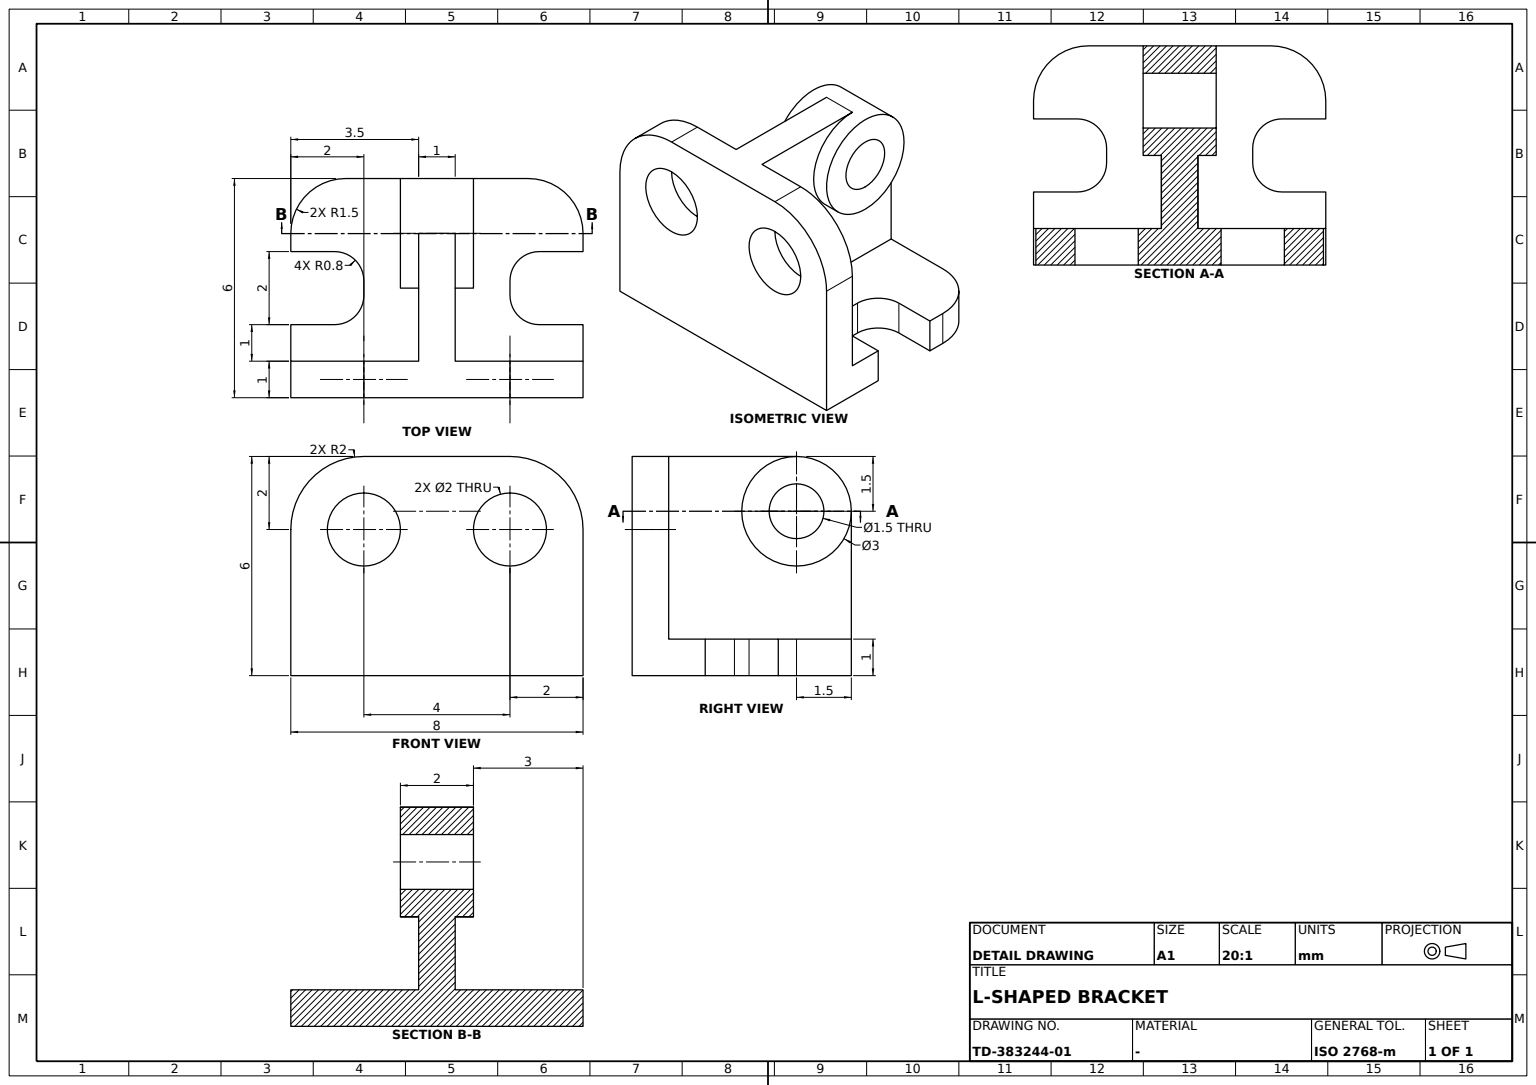
CATIA V5 part; units mm, degrees
sketch "Sketch1" plane through (0, 0, 0) normal (0, 0, 1) x (1, 0, 0)
  line L0 (4, 1.5) -> (4, 1)
  line L1 (4, -3) -> (-4, -3)
  line L2 (-4, -3) -> (-4, -1)
  line L3 (-2.5, 3) -> (2.5, 3)
  point P0 (4, 3)
  point P1 (4, -3)
  arc A0 (-4, 1.5) -> (-2.5, 3) centre (-2.5, 1.5) cw
  arc A1 (2.5, 3) -> (4, 1.5) centre (2.5, 1.5) cw
  point P2 (4, 0)
  line L4 (2, 0.2) -> (2, -0.2)
  point P3 (2, 0)
  line L5 (2.8, 1) -> (4, 1)
  line L6 (2.8, -1) -> (4, -1)
  point P4 (4, 1)
  point P5 (4, -1)
  arc A2 (2, 0.2) -> (2.8, 1) centre (2.8, 0.2) cw
  point P6 (2, 0.2)
  point P7 (2.8, 1)
  arc A3 (2, -0.2) -> (2.8, -1) centre (2.8, -0.2) ccw
  point P8 (2, -0.2)
  point P9 (2.8, -1)
  point P10 (-4, 1)
  point P11 (-2.8, 1)
  line L7 (-2.8, 1) -> (-4, 1)
  point P12 (-2, 0.2)
  arc A4 (-2, 0.2) -> (-2.8, 1) centre (-2.8, 0.2) ccw
  point P13 (-2, -0.2)
  line L8 (-2, 0.2) -> (-2, -0.2)
  point P14 (-2.8, -1)
  arc A5 (-2, -0.2) -> (-2.8, -1) centre (-2.8, -0.2) cw
  point P15 (-4, -1)
  line L9 (-2.8, -1) -> (-4, -1)
  line L10 (4, -1) -> (4, -3)
  line L11 (-4, 1) -> (-4, 1.5)
  dimension "length L1" = 8
  dimension "radius A0" = 1.5
  dimension "distance P0 P1" = 6
  dimension "radius A1" = 1.5
  dimension "radius A2" = 0.8
  dimension "radius A3" = 0.8
  constraint vertical L0 y-axis
  constraint vertical L2 y-axis
  constraint vertical L4 y-axis
  constraint vertical L10 y-axis
  constraint vertical L11 y-axis
  constraint horizontal L1 x-axis
  constraint horizontal L3 x-axis
  constraint horizontal L5 x-axis
  constraint horizontal L6 x-axis
  constraint equidistance L0 L2 origin
  constraint equidistance L1 L3 origin
  constraint tangency A0 L2
  constraint tangency A0 L3
  constraint tangency A1 L3
  constraint tangency A1 L0
  constraint tangency A2 L4
  constraint tangency A2 L5
  constraint tangency A3 L4
  constraint tangency A3 L6
  constraint coincidence L3 P0
  constraint coincidence L0 P0
  constraint coincidence P2 L0
  constraint coincidence P2 x-axis
  constraint coincidence P3 L4
  constraint coincidence L0 P5
  constraint coincidence L0 L10
  constraint coincidence L2 L11
  constraint symmetry P4 P10 y-axis
  constraint symmetry P7 P11 y-axis
  constraint symmetry L5 L7 y-axis
  constraint symmetry P6 P12 y-axis
  constraint symmetry A2 A4 y-axis
  constraint symmetry P8 P13 y-axis
  constraint symmetry L4 L8 y-axis
  constraint symmetry P9 P14 y-axis
  constraint symmetry A3 A5 y-axis
  constraint symmetry P5 P15 y-axis
  constraint symmetry L6 L9 y-axis
extrude "Pad1" add sketch "Sketch1" along normal blind 1
sketch "Sketch2" plane through (0, -3, 0) normal (0, -1, 0) x (1, 0, 0)
  point P0 (0, 3.5)
  line L0 (4, 4) -> (4, 1)
  line L1 (4, 1) -> (-4, 1)
  line L2 (-4, 1) -> (-4, 4)
  line L3 (-2, 6) -> (2, 6)
  point P1 (4, 6)
  point P2 (4, 1)
  line L4 (-4, 1) -> (4, 1) construction
  line L5 (-4, 0) -> (-4, 1) construction
  arc A0 (-4, 4) -> (-2, 6) centre (-2, 4) cw
  arc A1 (2, 6) -> (4, 4) centre (2, 4) cw
  dimension "length L1" = 8
  dimension "radius A0" = 2
  dimension "distance P1 P2" = 5
  dimension "radius A1" = 2
  constraint vertical L0 y-axis
  constraint vertical L2 y-axis
  constraint horizontal L1 x-axis
  constraint horizontal L3 x-axis
  constraint equidistance L0 L2 P0
  constraint equidistance L1 L3 P0
  constraint coincidence L4 L1
  constraint coincidence L5 L2
  constraint coincidence L3 P1
  constraint coincidence L0 P1
  constraint tangency A0 L2
  constraint tangency A0 L3
  constraint tangency A1 L3
  constraint tangency A1 L0
extrude "Pad2" add sketch "Sketch2" against normal blind 1
sketch "Sketch3" plane through (0, -2, 0) normal (0, 1, 0) x (-1, 0, 0)
  circle A0 centre (-2, 4) radius 1
  circle A1 centre (2, 4) radius 1
  arc A2 (-2, 6) -> (-4, 4) centre (-2, 4) ccw construction
  arc A3 (4, 4) -> (2, 6) centre (2, 4) ccw construction
  dimension "radius A1" = 1
  dimension "radius A0" = 1
  constraint concentricity A2 A0
  constraint concentricity A1 A3
extrude "Pocket1" cut sketch "Sketch3" against normal blind 1
sketch "Sketch4" plane through (0, 0, 0) normal (1, 0, 0) x (0, 1, 0)
  line L0 (-2, 6) -> (-2, 1)
  line L1 (-2, 1) -> (3, 1)
  line L2 (-2, 4) -> (-2, 6) construction
  line L3 (1.5, 1) -> (3, 1) construction
  line L4 (3, 1) -> (3, 4.5)
  line L5 (-2, 6) -> (1.5, 6)
  circle A0 centre (1.5, 4.5) radius 1.5
  point P0 (1.5, 6)
  point P1 (3, 4.5)
  dimension "length L0" = 5
  dimension "length L1" = 5
  dimension "radius A0" = 1.5
  dimension "distance A0 L5" = 0
  dimension "distance A0 L4" = 0
  constraint vertical L0 y-axis
  constraint vertical L4 y-axis
  constraint horizontal L1 x-axis
  constraint horizontal L5 x-axis
  constraint coincidence L2 L0
  constraint coincidence L1 L3
  constraint coincidence A0 P0
  constraint coincidence A0 P1
extrude "Pad3" add sketch "Sketch4" along normal mid plane 2 contours A0
extrude "Pad4" add sketch "Sketch4" along normal mid plane 1 contours L4 L1 L0 L5 material side at (0, 2.95, 2.75)
sketch "Sketch5" plane through (1, 0, 0) normal (1, 0, 0) x (0, 1, 0)
  circle A0 centre (1.5, 4.5) radius 0.75
  circle A1 centre (1.5, 4.5) radius 1.5 construction
  dimension "radius A0" = 0.75
  constraint concentricity A1 A0
extrude "Pocket2" cut sketch "Sketch5" against normal through all
